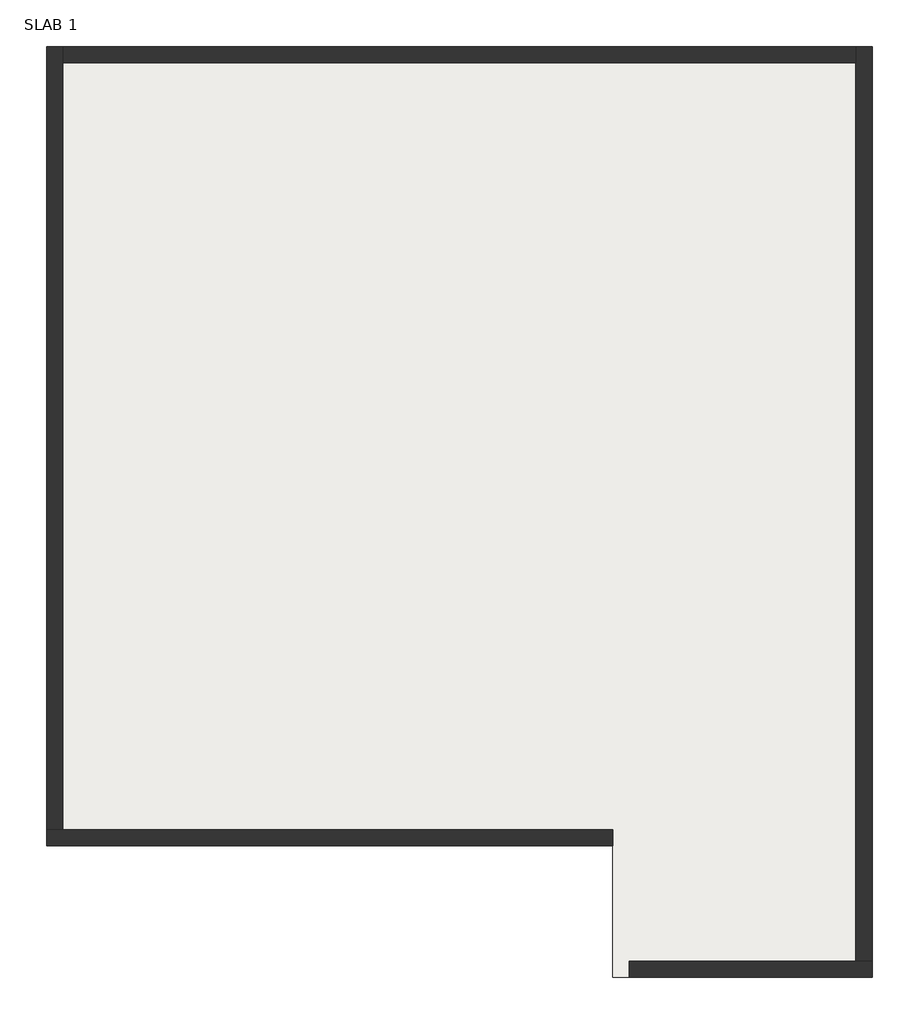
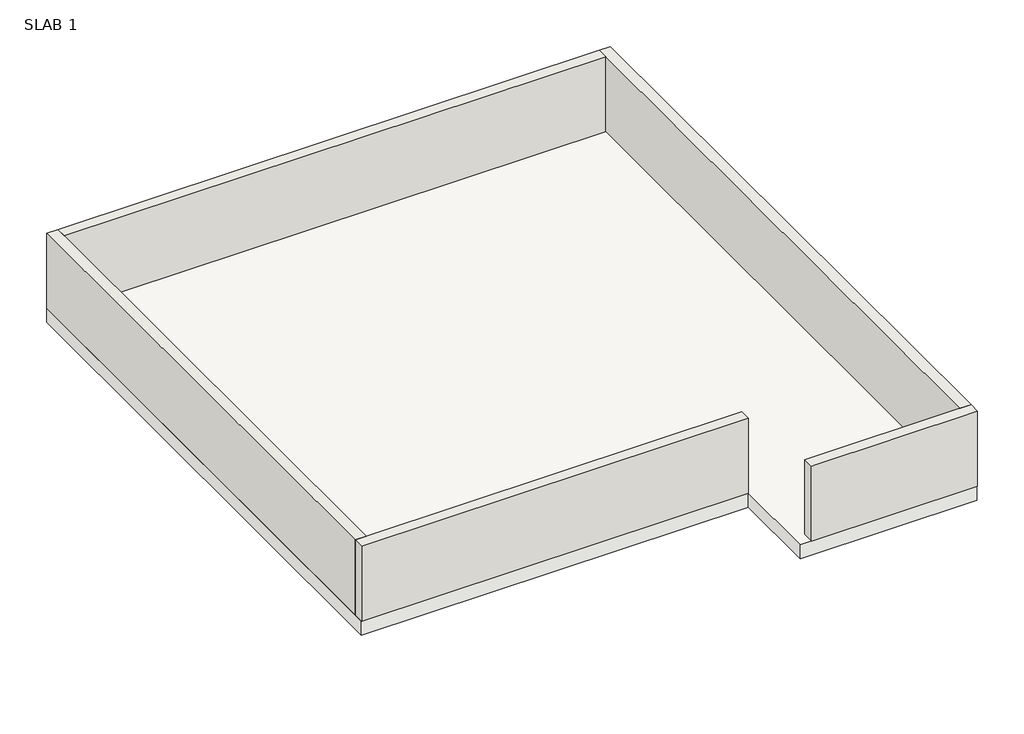
# One storey: 5 walls, 1 slab.
"""IFC4 building model written with IfcOpenShell, lengths in millimetres."""

from ifc_helpers import new_model, si_unit, frame, origin, place, context, project, spatial, polyline, outline, extrude, faceted_brep, element, save

model = new_model("IFC4")

# Units and contexts
model_context = context("Model", 3, world=origin())
ifc_project = project(units=[si_unit("LENGTHUNIT", "METRE", prefix="MILLI")], contexts=[model_context])

# Site, building, storey
site = spatial("IfcSite", under=ifc_project)
building = spatial("IfcBuilding", under=site)
storey = spatial("IfcBuildingStorey", under=building, Name="SLAB 1", Elevation=8737.6)

# Slab
placement = place(None, origin())
element("IfcSlab", 1, ObjectType="Generic - 12\"", at=placement, inside=storey, context=model_context, shape_type="SweptSolid", body=[
    extrude(outline(polyline([(3726.6918749, 13083.8953049), (3726.6918749, 53.6953049), (107.1918749, 53.6953049), (107.1918749, 1907.6881753), (-7817.6081251, 1907.6881753), (-7817.6081251, 13083.8953049), (3726.6918749, 13083.8953049)])), frame((0.0, 0.0, 8432.8), z_axis=(0.0, 0.0, 1.0), x_axis=(1.0, 0.0, 0.0)), (0.0, 0.0, 1.0), 304.8),
])

# Walls
element("IfcWall", 2, ObjectType="9\"", at=placement, inside=storey, context=model_context, shape_type="Brep", body=[
    faceted_brep([(335.8792748, 53.6953049, 8737.6), (3739.3918749, 53.6953049, 8737.6), (3739.3918749, 53.6953049, 10363.2), (335.8792748, 53.6953049, 10363.2), (335.8792748, 282.2953049, 8737.6), (335.8792748, 282.2953049, 10363.2), (3510.7918749, 282.2953049, 10363.2), (3739.3918749, 282.2953049, 10363.2), (3739.3918749, 282.2953049, 8737.6), (3510.7918749, 282.2953049, 8737.6)], [[[0, 1, 2, 3]], [[4, 5, 6, 7, 8, 9]], [[1, 0, 4, 9, 8]], [[3, 2, 7, 6, 5]], [[2, 1, 8, 7]], [[0, 3, 5, 4]]]),
])
element("IfcWall", 3, ObjectType="9\"", at=placement, inside=storey, context=model_context, shape_type="Brep", body=[
    faceted_brep([(3739.3918749, 282.2953049, 8737.6), (3739.3918749, 13083.8953049, 8737.6), (3739.3918749, 13083.8953049, 10363.2), (3739.3918749, 282.2953049, 10363.2), (3510.7918749, 282.2953049, 8737.6), (3510.7918749, 282.2953049, 10363.2), (3510.7918749, 12855.2953049, 10363.2), (3510.7918749, 13083.8953049, 10363.2), (3510.7918749, 13083.8953049, 8737.6), (3510.7918749, 12855.2953049, 8737.6)], [[[0, 1, 2, 3]], [[4, 5, 6, 7, 8, 9]], [[1, 0, 4, 9, 8]], [[3, 2, 7, 6, 5]], [[0, 3, 5, 4]], [[2, 1, 8, 7]]]),
])
element("IfcWall", 4, ObjectType="9\"", at=placement, inside=storey, context=model_context, shape_type="Brep", body=[
    faceted_brep([(107.2792748, 2123.7953049, 8737.6), (-7589.0081251, 2123.7953049, 8737.6), (-7817.6081251, 2123.7953049, 8737.6), (-7817.6081251, 2123.7953049, 10363.2), (-7589.0081251, 2123.7953049, 10363.2), (107.2792748, 2123.7953049, 10363.2), (107.2792748, 1895.1953049, 8737.6), (107.2792748, 1895.1953049, 10363.2), (-7817.6081251, 1895.1953049, 10363.2), (-7817.6081251, 1895.1953049, 8737.6)], [[[0, 1, 2, 3, 4, 5]], [[6, 7, 8, 9]], [[2, 1, 0, 6, 9]], [[5, 4, 3, 8, 7]], [[0, 5, 7, 6]], [[3, 2, 9, 8]]]),
])
element("IfcWall", 5, ObjectType="9\"", at=placement, inside=storey, context=model_context, shape_type="Brep", body=[
    faceted_brep([(-7589.0081251, 2123.7953049, 8737.6), (-7589.0081251, 12855.2953049, 8737.6), (-7589.0081251, 13083.8953049, 8737.6), (-7589.0081251, 13083.8953049, 10363.2), (-7589.0081251, 12855.2953049, 10363.2), (-7589.0081251, 2123.7953049, 10363.2), (-7817.6081251, 2123.7953049, 8737.6), (-7817.6081251, 2123.7953049, 10363.2), (-7817.6081251, 13083.8953049, 10363.2), (-7817.6081251, 13083.8953049, 8737.6)], [[[0, 1, 2, 3, 4, 5]], [[6, 7, 8, 9]], [[2, 1, 0, 6, 9]], [[5, 4, 3, 8, 7]], [[0, 5, 7, 6]], [[3, 2, 9, 8]]]),
])
element("IfcWall", 6, ObjectType="9\"", at=placement, inside=storey, context=model_context, shape_type="SweptSolid", body=[
    extrude(outline(polyline([(3510.7918749, 12855.2953049), (-7589.0081251, 12855.2953049), (-7589.0081251, 13083.8953049), (3510.7918749, 13083.8953049), (3510.7918749, 12855.2953049)])), frame((0.0, 0.0, 8737.6), z_axis=(0.0, 0.0, 1.0), x_axis=(1.0, 0.0, 0.0)), (0.0, 0.0, 1.0), 1625.6),
])

save(model, "model.ifc")

# Revit data of these elements
# Type "Generic - 12\""
#   Assembly Code = "B1010"
#   Function = 0
#   Layers, outside or top first: 1' - 0" no material (function 1)
# Type "9\""
#   Assembly Code = "B2010"
#   Layers, outside or top first: 0' - 9" "1 wall" (function 1)
# Element 1 (IfcSlab, "Generic - 12\"")
#   Height Offset From Level = 0' - 0"
#   Phase Created = New Construction
#   Materials on its faces: "Default Floor", "Acoustic Ceiling Tile 24 x 24"
# Elements 2, 4, 5, 6 (IfcWall, "9\"")
#   Top Offset = 0' - 0"
#   Base Offset = 0' - 0"
#   wall height = 5' - 4"
#   Phase Created = New Construction
#   Base Constraint = SLAB 1
#   Top Constraint = SLAB 2
#   Materials on its faces: "1 wall"
# Element 3 (IfcWall, "9\"")
#   Top Offset = 0' - 0"
#   Base Offset = 0' - 0"
#   wall height = 5' - 4"
#   Phase Created = New Construction
#   Base Constraint = SLAB 1
#   Top Constraint = SLAB 2
#   Materials on its faces: "1 wall", "Acoustic Ceiling Tile 24 x 24"
# Materials
#   "1 wall": class "Generic", colour RGB 172 157 136, transparency 0, Cost = 0
#   "Default Floor": colour RGB 128 128 128, transparency 0, Cost = 0
#   "Acoustic Ceiling Tile 24 x 24": class "Generic", colour RGB 232 232 232, transparency 0, Description = "Acoustic Ceiling Tile 24 x 24", Cost = 0
